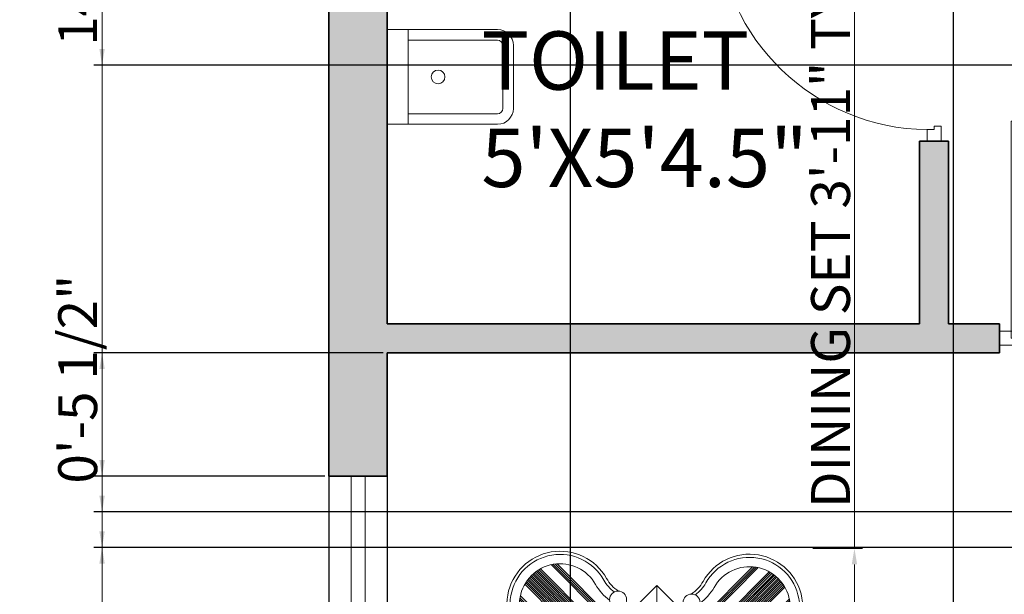
# Model space of a CAD drawing. Units: inches. Extents: x 2696 to 3240, y 1564 to 2310.
# Tile 39 of 76: x 2698 to 2850, y 1982 to 2071. Entities that reach past the tile are written whole.
import ezdxf

# ---------------------------------------------------------------- set-up
doc = ezdxf.new("R2010")
doc.units = ezdxf.units.IN
for name, color, linetype, lineweight in [('A-ANNO-DIMS', 3, 'Continuous', 18), ('A-AREA-IDEN', 7, 'Continuous', 18), ('A-DOOR', 4, 'Continuous', 18), ('A-FLOR-FIXT', 8, 'Continuous', 18), ('A-FURN', 251, 'Continuous', 13), ('A-WALL', 7, 'Continuous', 35), ('A-WALL-PATT', 9, 'Continuous', 13), ('WINDOW', 2, 'Continuous', 18)]:
    doc.layers.add(name, color=color, linetype=linetype, lineweight=lineweight)
doc.styles.add('TIMES NEW', font='times.ttf')
doc.styles.add('YQ_DIM', font='SUPEROS.SHX', dxfattribs={"width": 0.8, "bigfont": 'HZDX.SHX'})
doc.dimstyles.new('Siddhuu', dxfattribs={"dimtxt": 6, "dimasz": 2.5, "dimexe": 1.25, "dimexo": 0.625, "dimtad": 1, "dimdec": 1, "dimlunit": 4, "dimtxsty": 'TIMES NEW', "dimcen": 2.5, "dimclrd": 256, "dimclre": 1, "dimclrt": 7, "dimadec": 0, "dimazin": 0, "dimtfac": 1, "dimtdec": 1, "dimtmove": 0, "dimatfit": 3, "dimfxl": 1, "dimtolj": 1, "dimlwd": -1, "dimarcsym": 0})

# ---------------------------------------------------------------- blocks, each defined once
blk = doc.blocks.new('DR_D01')
for p, q in [((-0.45, 0.93), (-0.42, 0.93)), ((-0.45, 0.03), (-0.45, 0.93)), ((-0.42, 0.03), (-0.42, 0.93)), ((-0.5, 0.03), (-0.42, 0.03)), ((-0.5, 0.03), (-0.5, -0.03)), ((-0.45, 0.03), (-0.45, 0)), ((-0.45, 0), (-0.435, 0)), ((-0.435, 0), (-0.435, -0.03)), ((0.435, 0), (0.435, -0.03)), ((0.45, 0), (0.435, 0)), ((0.45, 0.03), (0.45, 0)), ((0.5, 0.03), (0.45, 0.03)), ((0.5, -0.03), (0.5, 0.03)), ((-0.435, -0.03), (-0.5, -0.03)), ((0.435, -0.03), (0.5, -0.03))]:
    blk.add_line(p, q)
blk.add_arc((-0.4602, 0.0206), 0.9103, 0.5915, 87.4664)
blk = doc.blocks.new('WD_WIN4')
for p, q in [((-0.5, 0.5), (0.5, 0.5)), ((-0.5, 0.12), (0.5, 0.12)), ((-0.5, -0.12), (0.5, -0.12)), ((-0.5, -0.5), (0.5, -0.5))]:
    blk.add_line(p, q)
blk = doc.blocks.new('WC')
at = {"layer": 'A-FURN'}
for p, q in [((0, 14.59), (-17.02, 14.59)), ((-3.24, 14.59), (-3.24, 0)), ((-19.45, 2.43), (-19.45, 12.16)), ((-17.83, 2.43), (-17.83, 12.16)), ((-3.24, 12.97), (-17.02, 12.97)), ((-3.24, 1.62), (-17.02, 1.62)), ((0, 0), (-17.02, 0))]:
    blk.add_line(p, q, dxfattribs=at)
blk.add_circle((-7.84, 7.3), 1.05, dxfattribs=at)
for centre, radius, start, end in [((-17.02, 12.16), 2.43, 90, 180), ((-17.02, 12.16), 0.811, 90, 180), ((-17.02, 2.43), 2.43, 180, 270), ((-17.02, 2.43), 0.811, 180, 270)]:
    blk.add_arc(centre, radius, start, end, dxfattribs=at)
blk = doc.blocks.new('DINING-SET-4')
h = blk.add_hatch()
h.set_pattern_fill('AR-CONC,_O', color=256, scale=0.03156, angle=135)
h.set_pattern_definition([(185, (694.1166, -47.9622), (-3.709933, 4.421326), [0.60121, -6.613307]), (130, (694.1166, -47.962), (-3.47714, -5.050095), [0.48097, -5.290645]), (235.451, (693.8074, -47.594), (-7.187067, -0.628735), [0.51095, -5.620443]), (181.1842, (692.983, -49.096), (-5.11118, 6.98761), [0.90181, -9.91996]), (231.6356, (692.557, -48.514), (-10.81945, -0.22364), [0.76642, -8.43066]), (126.184, (692.983, -49.096), (-10.81945, -0.22362), [0.72145, -7.93597]), (156, (692.6995, -48.2457), (-1.10128, 5.66559), [0.60121, -6.613307]), (101, (692.6995, -48.2457), (-5.48951, -2.73116), [0.48097, -5.290645]), (206.4514, (692.608, -47.7735), (-6.590787, 2.93441), [0.51095, -5.620443]), (172.5, (694.1166, -47.9622), (-1.955854, -1.8180035), [0, -5.226516, 0, -5.370807, 0, -5.310686]), (142.5, (694.1166, -47.9622), (-3.726774, -0.744482), [0, -3.062161, 0, -5.106274, 0, -2.024073]), (102.5, (695.3806, -49.2263), (-2.8979947, 3.15368), [0, -2.004032, 0, -6.25258, 0, -8.296694]), (92.5, (695.9475, -49.793), (-3.873065, 2.73823), [0, -2.605242, 0, -4.152355, 0, -5.891855])])
h.paths.add_polyline_path([(23.22, 8.74), (37.5, 23.02), (23.22, 37.31), (8.94, 23.02)])
for p, q in [((15.69, 35.33), (6.93, 44.09)), ((15.81, 35.56), (7.22, 44.15)), ((15.92, 35.79), (7.52, 44.19)), ((16.03, 36.02), (7.83, 44.22)), ((13.86, 32.79), (4.05, 42.6)), ((14.03, 32.97), (4.24, 42.76)), ((14.19, 33.15), (4.42, 42.91)), ((14.34, 33.33), (4.62, 43.06)), ((14.5, 33.52), (4.82, 43.2)), ((14.65, 33.71), (5.03, 43.33)), ((14.79, 33.91), (5.25, 43.45)), ((29.77, 35.57), (37.97, 43.77)), ((29.88, 35.34), (38.28, 43.74)), ((29.99, 35.11), (38.58, 43.7)), ((30.11, 34.88), (38.86, 43.64)), ((31, 33.46), (40.55, 43.01)), ((31.15, 33.26), (40.76, 42.88)), ((31.3, 33.07), (40.97, 42.75)), ((31.45, 32.88), (41.18, 42.61)), ((12.42, 31.5), (2.84, 41.08)), ((12.61, 31.65), (2.97, 41.3)), ((12.8, 31.8), (3.1, 41.5)), ((12.99, 31.96), (3.24, 41.7)), ((13.17, 32.12), (3.39, 41.89)), ((13.35, 32.28), (3.55, 42.08)), ((13.52, 32.45), (3.71, 42.26)), ((13.69, 32.62), (3.88, 42.43)), ((31.61, 32.7), (41.37, 42.46)), ((31.77, 32.52), (41.56, 42.31)), ((31.93, 32.34), (41.74, 42.15)), ((32.1, 32.17), (41.92, 41.98)), ((32.27, 32), (42.09, 41.81)), ((32.45, 31.83), (42.25, 41.63)), ((32.63, 31.67), (42.4, 41.45)), ((32.81, 31.51), (42.55, 41.25)), ((32.99, 31.35), (42.69, 41.05)), ((23.22, 38.2), (23.22, 40.88)), ((33.18, 31.2), (42.83, 40.85)), ((33.38, 31.05), (42.96, 40.63)), ((10.21, 30.19), (2.02, 38.38)), ((10.44, 30.3), (2.05, 38.7)), ((10.67, 30.41), (2.09, 39)), ((10.9, 30.53), (2.15, 39.28)), ((34.9, 30.08), (43.65, 38.83)), ((35.12, 29.96), (43.7, 38.55)), ((35.35, 29.85), (43.75, 38.25)), ((35.58, 29.74), (43.78, 37.94)), ((8.05, 23.02), (5.37, 23.02)), ((38.4, 23.02), (41.07, 23.02)), ((10.15, 15.95), (1.95, 7.75)), ((10.38, 15.84), (1.98, 7.44)), ((10.61, 15.73), (2.02, 7.14)), ((10.84, 15.61), (2.08, 6.86)), ((35.33, 15.7), (44.08, 6.94)), ((35.55, 15.81), (44.14, 7.23)), ((35.78, 15.93), (44.18, 7.52)), ((36.01, 16.03), (44.21, 7.83)), ((12.26, 14.72), (2.71, 5.17)), ((12.46, 14.57), (2.84, 4.95)), ((12.65, 14.42), (2.97, 4.75)), ((12.83, 14.27), (3.11, 4.54)), ((13.02, 14.11), (3.26, 4.35)), ((13.2, 13.95), (3.41, 4.16)), ((13.38, 13.78), (3.57, 3.98)), ((32.61, 13.7), (42.42, 3.89)), ((32.78, 13.87), (42.59, 4.06)), ((32.96, 14.03), (42.75, 4.24)), ((33.14, 14.19), (42.9, 4.43)), ((33.33, 14.35), (43.05, 4.63)), ((33.51, 14.5), (43.19, 4.83)), ((33.7, 14.65), (43.32, 5.04)), ((33.9, 14.8), (43.45, 5.25)), ((13.55, 13.62), (3.74, 3.8)), ((13.72, 13.45), (3.91, 3.63)), ((13.89, 13.27), (4.09, 3.47)), ((14.05, 13.09), (4.27, 3.32)), ((14.21, 12.91), (4.47, 3.17)), ((14.36, 12.72), (4.67, 3.03)), ((14.52, 12.54), (4.87, 2.89)), ((14.67, 12.34), (5.08, 2.76)), ((31.49, 12.43), (41.08, 2.85)), ((31.64, 12.62), (41.29, 2.97)), ((31.8, 12.81), (41.5, 3.11)), ((31.95, 12.99), (41.69, 3.25)), ((32.11, 13.18), (41.89, 3.4)), ((32.27, 13.35), (42.07, 3.55)), ((32.44, 13.53), (42.25, 3.72)), ((15.64, 10.82), (6.89, 2.07)), ((30.41, 10.68), (38.99, 2.1)), ((30.52, 10.91), (39.27, 2.15)), ((15.75, 10.6), (7.17, 2.02)), ((15.87, 10.37), (7.47, 1.97)), ((15.98, 10.14), (7.78, 1.94)), ((30.18, 10.22), (38.38, 2.03)), ((30.29, 10.45), (38.69, 2.06)), ((23.22, 7.85), (23.22, 5.17))]:
    blk.add_line(p, q)
for points in [[(41.07, 23.02), (23.22, 40.88), (5.37, 23.02), (23.22, 5.17)], [(38.4, 23.02), (23.22, 38.2), (8.05, 23.02), (23.22, 7.85)], [(37.5, 23.02), (23.22, 37.31), (8.94, 23.02), (23.22, 8.74)]]:
    blk.add_lwpolyline(points, close=True)
for centre in [(17.23, 38.71), (28.57, 38.26), (7.55, 29.03), (38.27, 28.51), (7.46, 17.15), (38.7, 17.23), (17.14, 7.47), (29.03, 7.55)]:
    blk.add_circle(centre, 1.31)
for centre, radius, start, end in [((8.28, 37.96), 8.21, 29.1881, 240.1532), ((8.28, 37.96), 7.72, 29.1881, 240.1532), ((37.51, 37.51), 8.21, 299.8468, 150.8119), ((8.28, 37.96), 6.28, 29.2752, 240.1505), ((37.51, 37.51), 7.72, 299.8468, 150.8119), ((37.51, 37.51), 6.28, 299.8495, 150.7248), ((20.45, 44.88), 7.72, 209.8594, 234.0675), ((20.45, 44.88), 6.28, 210.1015, 232.6572), ((20.45, 44.88), 5.79, 210.1015, 236.9513), ((25.34, 44.43), 5.79, 303.0487, 329.8985), ((25.34, 44.43), 6.28, 307.3428, 329.8985), ((25.34, 44.43), 7.72, 305.9325, 330.1406), ((5.4, 40.81), 11.66, 286.5158, 343.8317), ((40.4, 40.36), 11.66, 196.1683, 253.4842), ((1.37, 25.79), 7.72, 36.1055, 60.6071), ((44.43, 25.34), 7.72, 119.3929, 143.8945), ((1.37, 25.79), 5.79, 32.6748, 60.7093), ((1.37, 25.79), 6.28, 37.2611, 60.7093), ((44.43, 25.34), 6.28, 119.2907, 142.7389), ((44.43, 25.34), 5.79, 119.2907, 147.3252), ((1.29, 20.38), 5.79, 300.1015, 326.9513), ((44.87, 20.46), 5.79, 213.0487, 239.8985), ((8.21, 8.21), 8.21, 119.1881, 330.1532), ((1.29, 20.38), 6.28, 300.1015, 322.6572), ((1.29, 20.38), 7.72, 299.8594, 324.0675), ((5.36, 5.32), 11.66, 16.5158, 73.8317), ((40.8, 5.4), 11.66, 106.1683, 163.4842), ((37.95, 8.29), 8.21, 209.8468, 60.8119), ((44.87, 20.46), 7.72, 215.9325, 240.1406), ((44.87, 20.46), 6.28, 217.3428, 239.8985), ((8.21, 8.21), 7.72, 119.1881, 330.1532), ((8.21, 8.21), 6.28, 119.2752, 330.1505), ((37.95, 8.29), 7.72, 209.8468, 60.8119), ((37.95, 8.29), 6.28, 209.8495, 60.7248), ((25.78, 1.37), 7.72, 29.3929, 53.8945), ((20.38, 1.29), 7.72, 126.1055, 150.6071), ((20.38, 1.29), 6.28, 127.2611, 150.7093), ((20.38, 1.29), 5.79, 122.6748, 150.7093), ((25.78, 1.37), 5.79, 29.2907, 57.3252), ((25.78, 1.37), 6.28, 29.2907, 52.7389)]:
    blk.add_arc(centre, radius, start, end)
blk = doc.blocks.new('*D44')
at = {"layer": 'A-ANNO-DIMS', "transparency": 16777216}
for p, q in [((2826.68, 1989.07), (2826.68, 2086.33)), ((2826.68, 1944.45), (2826.68, 1986.57))]:
    blk.add_line(p, q, dxfattribs=at)
at = {"layer": 'A-ANNO-DIMS', "color": 1, "lineweight": -2, "transparency": 16777216}
for p, q in [((2820.24, 1989.07), (2827.93, 1989.07)), ((2820.24, 1941.95), (2827.93, 1941.95))]:
    blk.add_line(p, q, dxfattribs=at)
at = {"layer": 'A-ANNO-DIMS', "transparency": 16777216}
for points in [[(2826.26, 1986.57), (2827.09, 1986.57), (2826.68, 1989.07)], [(2826.26, 1944.45), (2827.09, 1944.45), (2826.68, 1941.95)]]:
    blk.add_solid(points, dxfattribs=at)
at = {"layer": 'Defpoints', "color": 0, "transparency": 16777216}
for p in [(2819.61, 1989.07), (2826.68, 1989.07), (2819.61, 1941.95)]:
    blk.add_point(p, dxfattribs=at)
at = {"layer": 'A-ANNO-DIMS', "color": 7, "transparency": 16777216, "insert": (2822.99, 2038.95), "char_height": 6, "attachment_point": 5, "rotation": 90, "style": 'TIMES NEW'}
blk.add_mtext('\\A1;DINING SET 3\'-11" TYP.', dxfattribs=at)
blk = doc.blocks.new('*D57')
at = {"layer": 'A-ANNO-DIMS', "color": 1, "lineweight": -2, "transparency": 16777216}
for p, q in [((2754.61, 2018.58), (2754.61, 1568.95)), ((2956.71, 2018.58), (2956.71, 1568.95))]:
    blk.add_line(p, q, dxfattribs=at)
at = {"layer": 'A-ANNO-DIMS', "transparency": 16777216}
blk.add_line((2757.11, 1570.2), (2954.21, 1570.2), dxfattribs=at)
for points in [[(2757.11, 1570.62), (2757.11, 1569.78), (2754.61, 1570.2)], [(2954.21, 1570.62), (2954.21, 1569.78), (2956.71, 1570.2)]]:
    blk.add_solid(points, dxfattribs=at)
at = {"layer": 'Defpoints', "color": 0, "transparency": 16777216}
for p in [(2754.61, 2019.2), (2956.71, 2019.2), (2956.71, 1570.2)]:
    blk.add_point(p, dxfattribs=at)
at = {"layer": 'A-ANNO-DIMS', "color": 7, "transparency": 16777216, "insert": (2855.66, 1573.88), "char_height": 6, "attachment_point": 5, "style": 'TIMES NEW'}
blk.add_mtext('\\A1;16\'-10"', dxfattribs=at)
blk = doc.blocks.new('*D58')
at = {"layer": 'A-ANNO-DIMS', "color": 1, "lineweight": -2, "transparency": 16777216}
for p, q in [((2753.99, 2019.2), (2709.36, 2019.2)), ((2753.99, 1911.2), (2709.36, 1911.2))]:
    blk.add_line(p, q, dxfattribs=at)
at = {"layer": 'A-ANNO-DIMS', "transparency": 16777216}
blk.add_line((2710.61, 1913.7), (2710.61, 2016.7), dxfattribs=at)
for points in [[(2710.19, 2016.7), (2711.03, 2016.7), (2710.61, 2019.2)], [(2710.19, 1913.7), (2711.03, 1913.7), (2710.61, 1911.2)]]:
    blk.add_solid(points, dxfattribs=at)
at = {"layer": 'Defpoints', "color": 0, "transparency": 16777216}
for p in [(2710.61, 2019.2), (2754.61, 2019.2), (2754.61, 1911.2)]:
    blk.add_point(p, dxfattribs=at)
at = {"layer": 'A-ANNO-DIMS', "color": 7, "transparency": 16777216, "insert": (2706.93, 1965.2), "char_height": 6, "attachment_point": 5, "rotation": 90, "style": 'TIMES NEW'}
blk.add_mtext('\\A1;9\'-0"', dxfattribs=at)
blk = doc.blocks.new('*D62')
at = {"layer": 'A-ANNO-DIMS', "color": 1, "lineweight": -2, "transparency": 16777216}
for p, q in [((2965.08, 2140.7), (2709.36, 2140.7)), ((2965.08, 2063.59), (2709.36, 2063.59))]:
    blk.add_line(p, q, dxfattribs=at)
at = {"layer": 'A-ANNO-DIMS', "transparency": 16777216}
blk.add_line((2710.61, 2066.09), (2710.61, 2138.2), dxfattribs=at)
for points in [[(2710.19, 2138.2), (2711.03, 2138.2), (2710.61, 2140.7)], [(2710.19, 2066.09), (2711.03, 2066.09), (2710.61, 2063.59)]]:
    blk.add_solid(points, dxfattribs=at)
at = {"layer": 'Defpoints', "color": 0, "transparency": 16777216}
for p in [(2710.61, 2140.7), (2965.71, 2140.7), (2965.71, 2063.59)]:
    blk.add_point(p, dxfattribs=at)
at = {"layer": 'A-ANNO-DIMS', "color": 7, "transparency": 16777216, "insert": (2706.93, 2102.15), "char_height": 6, "attachment_point": 5, "rotation": 90, "style": 'TIMES NEW'}
blk.add_mtext('\\A1;6\'-5"', dxfattribs=at)
blk = doc.blocks.new('*D64')
at = {"layer": 'A-ANNO-DIMS', "color": 1, "lineweight": -2, "transparency": 16777216}
for p, q in [((3073.08, 2206.7), (2709.36, 2206.7)), ((3068.58, 1989.2), (2709.36, 1989.2))]:
    blk.add_line(p, q, dxfattribs=at)
at = {"layer": 'A-ANNO-DIMS', "transparency": 16777216}
blk.add_line((2710.61, 1991.7), (2710.61, 2204.2), dxfattribs=at)
for points in [[(2710.19, 2204.2), (2711.03, 2204.2), (2710.61, 2206.7)], [(2710.19, 1991.7), (2711.03, 1991.7), (2710.61, 1989.2)]]:
    blk.add_solid(points, dxfattribs=at)
at = {"layer": 'Defpoints', "color": 0, "transparency": 16777216}
for p in [(2710.61, 2206.7), (3073.71, 2206.7), (3069.21, 1989.2)]:
    blk.add_point(p, dxfattribs=at)
at = {"layer": 'A-ANNO-DIMS', "color": 7, "transparency": 16777216, "insert": (2706.85, 2097.95), "char_height": 6, "attachment_point": 5, "rotation": 90, "style": 'TIMES NEW'}
blk.add_mtext('\\A1;18\'-1 1/2"', dxfattribs=at)
blk = doc.blocks.new('*D68')
at = {"layer": 'A-ANNO-DIMS', "color": 1, "lineweight": -2, "transparency": 16777216}
for p, q in [((2745.61, 2261.58), (2745.61, 1568.95)), ((2782.83, 2261.58), (2782.83, 1568.95))]:
    blk.add_line(p, q, dxfattribs=at)
at = {"layer": 'A-ANNO-DIMS', "transparency": 16777216}
blk.add_line((2748.11, 1570.2), (2780.33, 1570.2), dxfattribs=at)
for points in [[(2748.11, 1570.62), (2748.11, 1569.78), (2745.61, 1570.2)], [(2780.33, 1570.62), (2780.33, 1569.78), (2782.83, 1570.2)]]:
    blk.add_solid(points, dxfattribs=at)
at = {"layer": 'Defpoints', "color": 0, "transparency": 16777216}
for p in [(2745.61, 2262.2), (2782.83, 2262.2), (2782.83, 1570.2)]:
    blk.add_point(p, dxfattribs=at)
at = {"layer": 'A-ANNO-DIMS', "color": 7, "transparency": 16777216, "insert": (2764.22, 1573.88), "char_height": 6, "attachment_point": 5, "style": 'TIMES NEW'}
blk.add_mtext('\\A1;3\'-1"', dxfattribs=at)
blk = doc.blocks.new('*D69')
at = {"layer": 'A-ANNO-DIMS', "color": 1, "lineweight": -2, "transparency": 16777216}
for p, q in [((2841.89, 2261.58), (2841.89, 1568.95)), ((2905.91, 2261.58), (2905.91, 1568.95))]:
    blk.add_line(p, q, dxfattribs=at)
at = {"layer": 'A-ANNO-DIMS', "transparency": 16777216}
blk.add_line((2844.39, 1570.2), (2903.41, 1570.2), dxfattribs=at)
for points in [[(2844.39, 1570.62), (2844.39, 1569.78), (2841.89, 1570.2)], [(2903.41, 1570.62), (2903.41, 1569.78), (2905.91, 1570.2)]]:
    blk.add_solid(points, dxfattribs=at)
at = {"layer": 'Defpoints', "color": 0, "transparency": 16777216}
for p in [(2841.89, 2262.2), (2905.91, 2262.2), (2905.91, 1570.2)]:
    blk.add_point(p, dxfattribs=at)
at = {"layer": 'A-ANNO-DIMS', "color": 7, "transparency": 16777216, "insert": (2873.9, 1573.88), "char_height": 6, "attachment_point": 5, "style": 'TIMES NEW'}
blk.add_mtext('\\A1;5\'-4"', dxfattribs=at)
blk = doc.blocks.new('*D72')
at = {"layer": 'A-ANNO-DIMS', "color": 1, "lineweight": -2, "transparency": 16777216}
for p, q in [((2744.99, 2169.67), (2709.36, 2169.67)), ((2744.99, 2000.2), (2709.36, 2000.2))]:
    blk.add_line(p, q, dxfattribs=at)
at = {"layer": 'A-ANNO-DIMS', "transparency": 16777216}
blk.add_line((2710.61, 2167.17), (2710.61, 2002.7), dxfattribs=at)
for points in [[(2710.19, 2167.17), (2711.03, 2167.17), (2710.61, 2169.67)], [(2710.19, 2002.7), (2711.03, 2002.7), (2710.61, 2000.2)]]:
    blk.add_solid(points, dxfattribs=at)
at = {"layer": 'Defpoints', "color": 0, "transparency": 16777216}
for p in [(2745.61, 2169.67), (2710.61, 2000.2), (2745.61, 2000.2)]:
    blk.add_point(p, dxfattribs=at)
at = {"layer": 'A-ANNO-DIMS', "color": 7, "transparency": 16777216, "insert": (2706.85, 2084.94), "char_height": 6, "attachment_point": 5, "rotation": 90, "style": 'TIMES NEW'}
blk.add_mtext('\\A1;14\'-1 1/2"', dxfattribs=at)
blk = doc.blocks.new('*D77')
at = {"layer": 'A-ANNO-DIMS', "transparency": 16777216}
for p, q in [((2710.61, 1997.2), (2710.61, 2030.6)), ((2710.61, 1989.2), (2710.61, 1994.7)), ((2710.61, 1986.7), (2710.61, 1984.2))]:
    blk.add_line(p, q, dxfattribs=at)
at = {"layer": 'A-ANNO-DIMS', "color": 1, "lineweight": -2, "transparency": 16777216}
for p, q in [((3189.99, 1994.7), (2709.36, 1994.7)), ((3189.99, 1989.2), (2709.36, 1989.2))]:
    blk.add_line(p, q, dxfattribs=at)
at = {"layer": 'A-ANNO-DIMS', "transparency": 16777216}
for points in [[(2710.19, 1997.2), (2711.03, 1997.2), (2710.61, 1994.7)], [(2710.19, 1986.7), (2711.03, 1986.7), (2710.61, 1989.2)]]:
    blk.add_solid(points, dxfattribs=at)
at = {"layer": 'Defpoints', "color": 0, "transparency": 16777216}
for p in [(2710.61, 1994.7), (3190.61, 1994.7), (3190.61, 1989.2)]:
    blk.add_point(p, dxfattribs=at)
at = {"layer": 'A-ANNO-DIMS', "color": 7, "transparency": 16777216, "insert": (2706.85, 2015.15), "char_height": 6, "attachment_point": 5, "rotation": 90, "style": 'TIMES NEW'}
blk.add_mtext('\\A1;0\'-5 1/2"', dxfattribs=at)

msp = doc.modelspace()

# ---------------------------------------------------------------- hatches: boundary and pattern name
at = {"layer": 'A-WALL-PATT', "transparency": 33554556}
h = msp.add_hatch(color=256, dxfattribs=at)
h.dxf.hatch_style = 1
h.paths.add_polyline_path([(2879.11, 2253.2), (2905.91, 2253.2), (2905.91, 2262.2), (2841.89, 2262.2), (2841.89, 2253.2), (2870.11, 2253.2), (2870.11, 2176.6), (2965.71, 2176.6), (2965.71, 2206.7), (2973.58, 2206.7), (2973.58, 2215.7), (2965.71, 2215.7), (2965.71, 2262.2), (2929.91, 2262.2), (2929.91, 2253.2), (2956.71, 2253.2), (2956.71, 2185.6), (2879.11, 2185.6)])
h.paths.add_polyline_path([(2782.83, 2262.2), (2745.61, 2262.2), (2745.61, 2228.73), (2754.61, 2228.73), (2754.61, 2253.2), (2782.83, 2253.2)])
h.paths.add_polyline_path([(2754.61, 2136.2), (2965.71, 2136.2), (2965.71, 2145.2), (2879.11, 2145.2), (2879.11, 2147.07), (2877.34, 2147.07), (2870.11, 2147.07), (2870.11, 2145.2), (2754.61, 2145.2), (2754.61, 2169.67), (2745.61, 2169.67), (2745.61, 2000.2), (2754.61, 2000.2), (2754.61, 2019.2), (2849.08, 2019.2), (2849.08, 2023.7), (2841.21, 2023.7), (2841.21, 2051.83), (2836.71, 2051.83), (2836.71, 2023.7), (2754.61, 2023.7), (2754.61, 2091.2), (2836.71, 2091.2), (2836.71, 2087.83), (2841.21, 2087.83), (2841.21, 2095.7), (2754.61, 2095.7)])
h.paths.add_polyline_path([(2965.71, 2136.2), (2956.71, 2136.2), (2956.71, 2023.7), (2885.08, 2023.7), (2885.08, 2019.2), (2956.71, 2019.2), (2956.71, 1950.58), (2965.71, 1950.58), (2965.71, 1980.2), (2973.58, 1980.2), (2973.58, 1989.2), (2965.71, 1989.2)])
h.paths.add_polyline_path([(2754.61, 1906.7), (2880.21, 1906.7), (2884.71, 1906.7), (2956.71, 1906.7), (2956.71, 1792.7), (2944.71, 1792.7), (2944.71, 1783.7), (2956.71, 1783.7), (2956.71, 1740.2), (2884.71, 1740.2), (2884.71, 1783.7), (2896.71, 1783.7), (2896.71, 1792.7), (2884.71, 1792.7), (2884.71, 1846.7), (2880.21, 1846.7), (2880.21, 1740.2), (2754.61, 1740.2), (2754.61, 1777.2), (2745.61, 1777.2), (2745.61, 1692.7), (2754.61, 1692.7), (2754.61, 1731.2), (2956.71, 1731.2), (2956.71, 1723.33), (2965.71, 1723.33), (2965.71, 1884.2), (2973.58, 1884.2), (2973.58, 1893.2), (2965.71, 1893.2), (2965.71, 1914.58), (2956.71, 1914.58), (2956.71, 1911.2), (2754.61, 1911.2), (2754.61, 1930.2), (2745.61, 1930.2), (2745.61, 1817.2), (2754.61, 1817.2), (2754.61, 1854.2), (2826.61, 1854.2), (2826.61, 1868.83), (2822.11, 1868.83), (2822.11, 1858.7), (2754.61, 1858.7)])
h.paths.add_polyline_path([(2965.71, 1656.2), (3008.24, 1656.2), (3008.24, 1665.2), (2965.71, 1665.2), (2965.71, 1693.33), (2956.71, 1693.33), (2956.71, 1686.2), (2934.58, 1686.2), (2934.58, 1681.7), (2956.71, 1681.7), (2956.71, 1614.2), (2896.71, 1614.2), (2896.71, 1681.7), (2904.58, 1681.7), (2904.58, 1686.2), (2892.21, 1686.2), (2892.21, 1614.2), (2858.41, 1614.2), (2858.41, 1605.2), (2965.71, 1605.2)])
h.paths.add_polyline_path([(2788.41, 1614.2), (2754.61, 1614.2), (2754.61, 1652.7), (2745.61, 1652.7), (2745.61, 1605.2), (2788.41, 1605.2)])
h.paths.add_polyline_path([(3199.61, 1633.05), (3190.61, 1633.05), (3190.61, 1614.2), (3082.61, 1614.2), (3082.61, 1665.2), (3070.24, 1665.2), (3070.24, 1656.2), (3078.11, 1656.2), (3078.11, 1605.2), (3199.61, 1605.2)])
h.paths.add_polyline_path([(3199.61, 1702.05), (3190.61, 1702.05), (3190.61, 1699.7), (3106.61, 1699.7), (3106.61, 1747.7), (3190.61, 1747.7), (3190.61, 1752.2), (3082.61, 1752.2), (3082.61, 1760.08), (3078.11, 1760.08), (3078.11, 1747.7), (3102.11, 1747.7), (3102.11, 1699.7), (3078.11, 1699.7), (3078.11, 1695.2), (3190.61, 1695.2), (3190.61, 1676.35), (3199.61, 1676.35)])
h.paths.add_polyline_path([(3199.61, 1783.2), (3190.61, 1783.2), (3190.61, 1745.35), (3199.61, 1745.35)])
h.paths.add_polyline_path([(3082.61, 1884.2), (3190.61, 1884.2), (3190.61, 1853.2), (3199.61, 1853.2), (3199.61, 1901.7), (3190.61, 1901.7), (3190.61, 1893.2), (3005.58, 1893.2), (3005.58, 1891.28), (3005.58, 1884.2), (3078.11, 1884.2), (3078.11, 1792.08), (3082.61, 1792.08)])
h.paths.add_polyline_path([(3199.61, 1994.7), (3190.61, 1994.7), (3190.61, 1989.2), (3073.71, 1989.2), (3073.71, 2034.2), (3069.21, 2034.2), (3069.21, 1989.2), (3005.58, 1989.2), (3005.58, 1980.2), (3190.61, 1980.2), (3190.61, 1971.7), (3199.61, 1971.7)])
h.paths.add_polyline_path([(3199.61, 2155.2), (3190.61, 2155.2), (3190.61, 2064.7), (3199.61, 2064.7)])
h.paths.add_polyline_path([(3190.61, 2074.7), (3106.61, 2074.7), (3106.61, 2122.7), (3190.61, 2122.7), (3190.61, 2127.2), (3082.71, 2127.2), (3082.71, 2135.08), (3073.71, 2135.08), (3073.71, 2122.7), (3102.11, 2122.7), (3102.11, 2074.7), (3069.21, 2074.7), (3069.21, 2070.2), (3190.61, 2070.2)])
h.paths.add_polyline_path([(3082.71, 2253.2), (3190.61, 2253.2), (3190.61, 2225.2), (3199.61, 2225.2), (3199.61, 2262.2), (3073.71, 2262.2), (3073.71, 2215.7), (3035.58, 2215.7), (3035.58, 2206.7), (3073.71, 2206.7), (3073.71, 2171.08), (3082.71, 2171.08)])

# ---------------------------------------------------------------- linework, layer by layer
at = {"layer": 'A-WALL'}
for p, q in [((2745.61, 2000.2), (2745.61, 2169.67)), ((2754.61, 2023.7), (2754.61, 2091.2)), ((2836.71, 2051.83), (2836.71, 2023.7)), ((2841.21, 2051.83), (2836.71, 2051.83)), ((2841.21, 2051.83), (2841.21, 2023.7)), ((2754.61, 2023.7), (2836.71, 2023.7)), ((2841.21, 2023.7), (2849.08, 2023.7)), ((2849.08, 2023.7), (2849.08, 2019.2)), ((2754.61, 2019.2), (2849.08, 2019.2)), ((2754.61, 2000.2), (2754.61, 2019.2)), ((2754.61, 2000.2), (2745.61, 2000.2))]:
    msp.add_line(p, q, dxfattribs=at)

# ---------------------------------------------------------------- block references
at = {"layer": 'A-DOOR', "xscale": 36, "yscale": -36, "zscale": 36, "rotation": 270.0000000000007}
msp.add_blockref('DR_D01', (2838.96, 2069.83), dxfattribs=at)
at = {"layer": 'A-DOOR', "xscale": 36, "yscale": 36, "zscale": 36}
msp.add_blockref('DR_D01', (2867.08, 2021.45), dxfattribs=at)
at = {"layer": 'A-FLOR-FIXT', "xscale": -1}
msp.add_blockref('WC', (2754.61, 2054.46), dxfattribs=at)
at = {"layer": 'A-FURN'}
msp.add_blockref('DINING-SET-4', (2772.99, 1942.44), dxfattribs=at)
at = {"layer": 'WINDOW', "xscale": 70, "yscale": 8.999999999999545, "zscale": 70, "rotation": 270}
msp.add_blockref('WD_WIN4', (2750.11, 1965.2), dxfattribs=at)

# ---------------------------------------------------------------- texts
at = {"layer": 'A-AREA-IDEN', "insert": (2769.13, 2068.78), "char_height": 9, "attachment_point": 1, "style": 'YQ_DIM'}
msp.add_mtext_dynamic_manual_height_columns('TOILET\\P5\'X5\'4.5"', width=48.0032, gutter_width=12.5, heights=[0], dxfattribs=at)

# ---------------------------------------------------------------- dimensions: what is measured, and where the dimension line sits
at = {"layer": 'A-ANNO-DIMS'}
for base, p1, p2, picture, middle in [((2782.83, 1570.2), (2745.61, 2262.2), (2782.83, 2262.2), '*D68', (2764.22, 1573.88)), ((2905.91, 1570.2), (2841.89, 2262.2), (2905.91, 2262.2), '*D69', (2873.9, 1573.88)), ((2956.71, 1570.2), (2754.61, 2019.2), (2956.71, 2019.2), '*D57', (2855.66, 1573.88))]:
    dim = msp.add_linear_dim(base=base, p1=p1, p2=p2, dimstyle='Siddhuu', override={"dimdec": 1, "dimlfac": 1, "dimrnd": 0, "dimzin": 1, "dimdsep": 46, "dimlunit": 4, "dimfrac": 2}, dxfattribs=at)
    dim.commit()
    dim.dimension.update_dxf_attribs({"geometry": picture, "text_midpoint": middle})
for base, p1, p2, picture, middle in [((2710.61, 2206.7), (3069.21, 1989.2), (3073.71, 2206.7), '*D64', (2706.85, 2097.95)), ((2710.61, 2000.2), (2745.61, 2169.67), (2745.61, 2000.2), '*D72', (2706.85, 2084.94)), ((2710.61, 2140.7), (2965.71, 2063.59), (2965.71, 2140.7), '*D62', (2706.93, 2102.15)), ((2710.61, 1994.7), (3190.61, 1989.2), (3190.61, 1994.7), '*D77', (2706.85, 2015.15)), ((2710.61, 2019.2), (2754.61, 1911.2), (2754.61, 2019.2), '*D58', (2706.93, 1965.2))]:
    dim = msp.add_linear_dim(base=base, p1=p1, p2=p2, angle=90, dimstyle='Siddhuu', override={"dimdec": 1, "dimlfac": 1, "dimrnd": 0, "dimzin": 1, "dimdsep": 46, "dimlunit": 4, "dimfrac": 2}, dxfattribs=at)
    dim.commit()
    dim.dimension.update_dxf_attribs({"geometry": picture, "text_midpoint": middle})
dim = msp.add_linear_dim(base=(2826.68, 1989.07), p1=(2819.61, 1941.95), p2=(2819.61, 1989.07), angle=90, text='DINING SET <> TYP.', dimstyle='Siddhuu', override={"dimdec": 1, "dimlfac": 1, "dimrnd": 0, "dimzin": 1, "dimdsep": 46, "dimlunit": 4, "dimfrac": 2}, dxfattribs=at)
dim.commit()
dim.dimension.update_dxf_attribs({"geometry": '*D44', "text_midpoint": (2822.99, 2038.95)})

doc.saveas('drawing.dxf')
